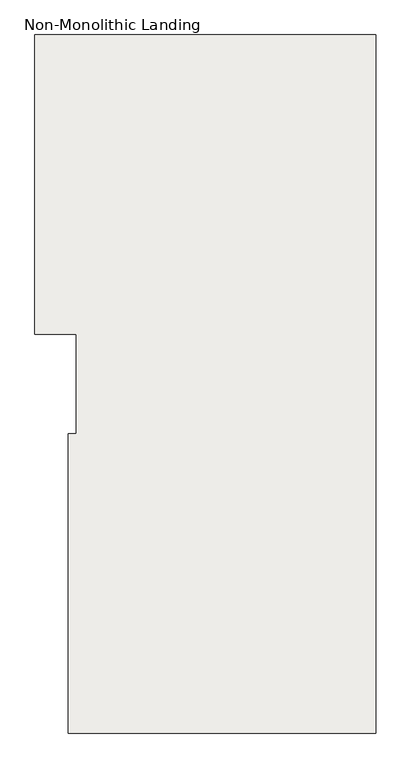
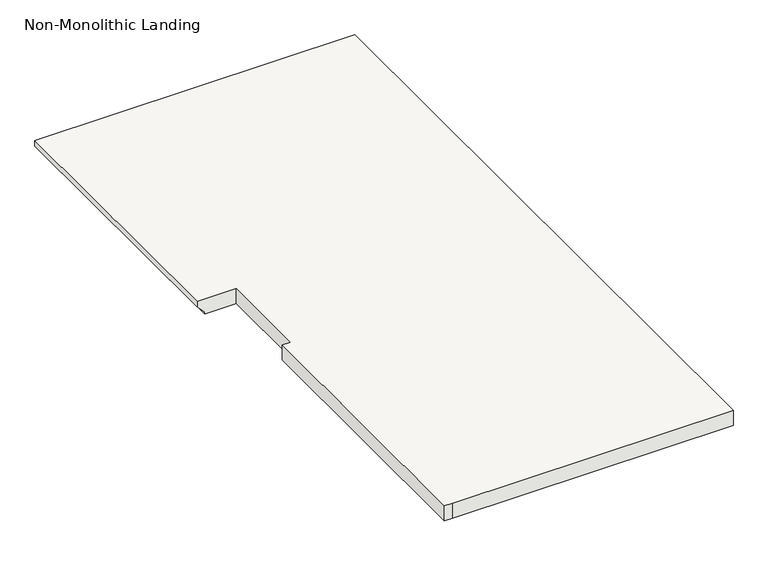
"""IFC4 building model written with IfcOpenShell, lengths in millimetres: slab geometry, Non-Monolithic Landing."""

from ifc_helpers import new_model, si_unit, origin, place, context, project, spatial, faceted_brep, source, transform, mapped, element, save


def non_monolithic_landing_135adda5(model_context):
    return source(origin(), model_context, "Body", "Brep", [
        faceted_brep([(551.235938, 2339.7857363, 1488.0166667), (551.235938, 2339.7857363, 1507.0666667), (551.235938, 3254.1857363, 1507.0666667), (551.235938, 3254.1857363, 1488.0166667), (576.635938, 2339.7857363, 1462.6166667), (576.635938, 3254.1857363, 1462.6166667), (678.235938, 2339.7857363, 1507.0666667), (678.235938, 2034.9857363, 1507.0666667), (652.835938, 2034.9857363, 1507.0666667), (652.835938, 1120.5857363, 1507.0666667), (678.235938, 1120.5857363, 1507.0666667), (1592.635938, 1120.5857363, 1507.0666667), (1592.635938, 3254.1857363, 1507.0666667), (576.635938, 2339.7857363, 1456.2666667), (576.635938, 3254.1857363, 1456.2666667), (1592.635938, 3254.1857363, 1456.2666667), (1592.635938, 1120.5857363, 1456.2666667), (678.235938, 1120.5857363, 1456.2666667), (652.835938, 1120.5857363, 1456.2666667), (652.835938, 2034.9857363, 1456.2666667), (678.235938, 2034.9857363, 1456.2666667), (678.235938, 2339.7857363, 1456.2666667)], [[[0, 1, 2, 3]], [[4, 0, 3, 5]], [[6, 7, 8, 9, 10, 11, 12, 2, 1]], [[13, 14, 15, 16, 17, 18, 19, 20, 21]], [[14, 13, 4, 5]], [[6, 1, 0, 4, 13, 21]], [[7, 6, 21, 20]], [[8, 7, 20, 19]], [[9, 8, 19, 18]], [[10, 9, 18, 17]], [[11, 10, 17, 16]], [[12, 11, 16, 15]], [[2, 12, 15, 14, 5, 3]]]),
    ])


if __name__ == "__main__":
    model = new_model("IFC4")
    model_context = context("Model", 3, world=origin())
    ifc_project = project(units=[si_unit("LENGTHUNIT", "METRE", prefix="MILLI")], contexts=[model_context])
    site = spatial("IfcSite", under=ifc_project)
    building = spatial("IfcBuilding", under=site)
    placement = place(None, origin())
    non_monolithic_landing_shape = non_monolithic_landing_135adda5(model_context)
    element("IfcSlab", 1, ObjectType="Non-Monolithic Landing", at=placement, inside=building, context=model_context, shape_type="MappedRepresentation", body=[
        mapped(non_monolithic_landing_shape, transform((0.0, 0.0, 0.0), x_axis=(1.0, 0.0, 0.0), y_axis=(0.0, 1.0, 0.0), z_axis=(0.0, 0.0, 1.0))),
    ])
    save(model, "model.ifc")

# Revit data of these elements
# Element 1 (IfcSlab, "Non-Monolithic Landing")
#   Materials on its faces: "BURGUNDY COLOUR"
# Materials
#   "BURGUNDY COLOUR": class "Generic", colour RGB 120 120 120, transparency 0, Cost = 0
